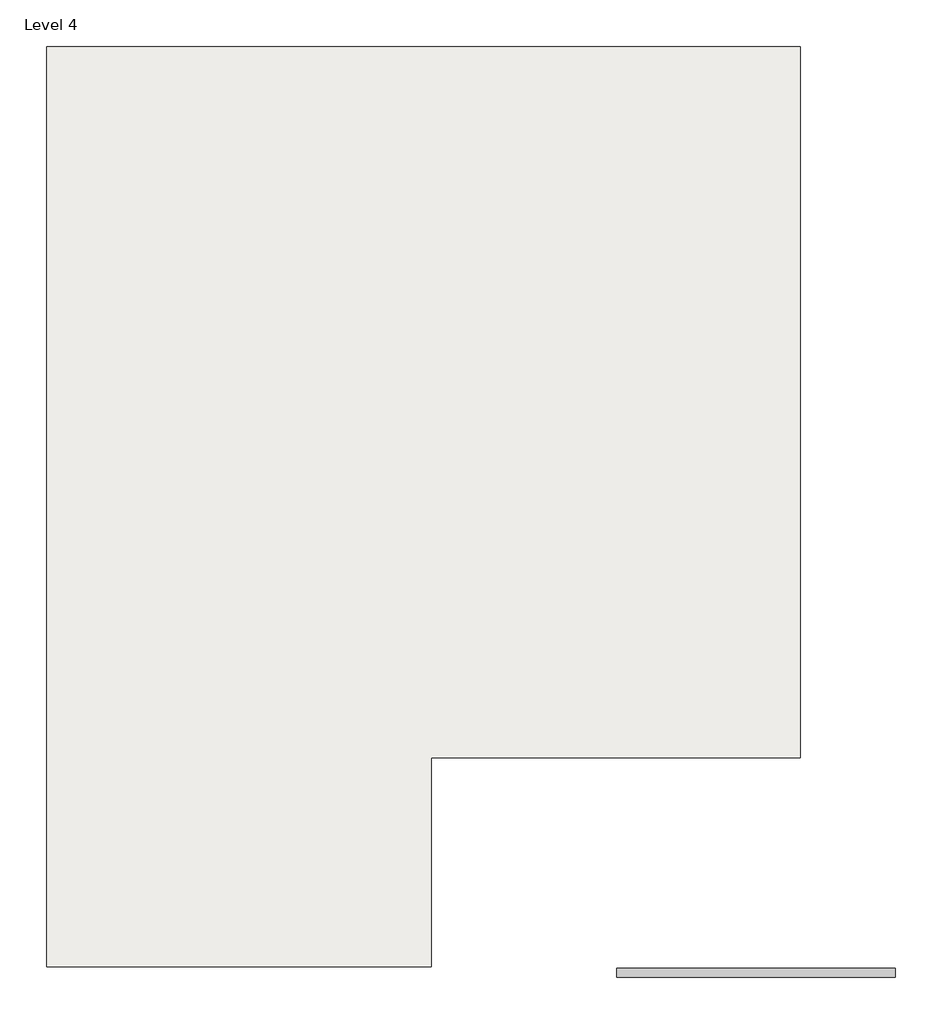
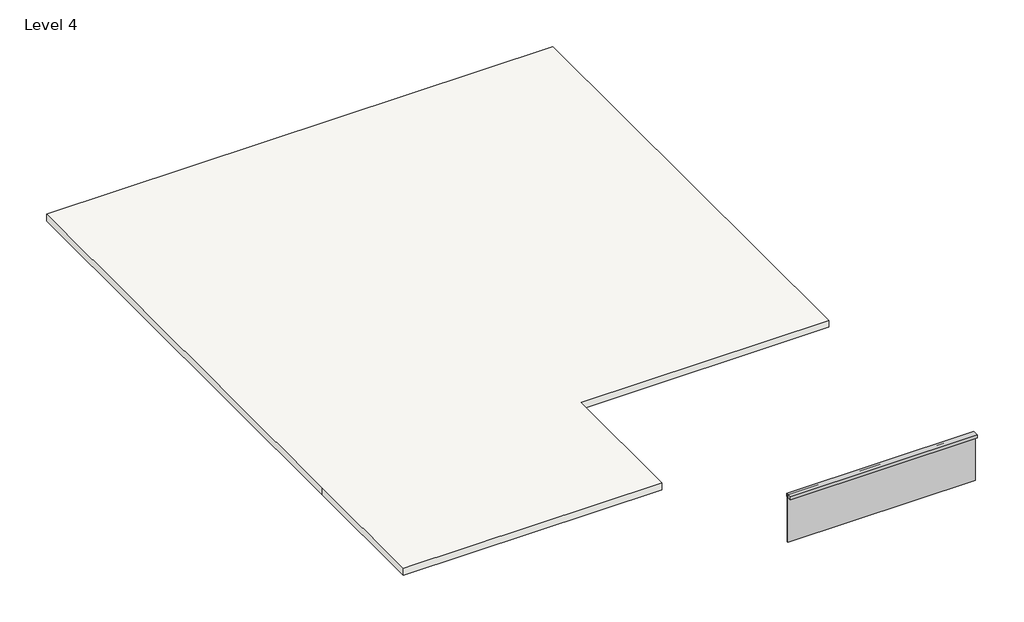
# One storey: 1 member, 1 plate, 1 slab.
"""IFC4 building model written with IfcOpenShell, lengths in millimetres."""

from ifc_helpers import new_model, si_unit, frame, origin, place, context, project, spatial, polyline, outline, extrude, transform, mapped, element, save
from components import member_63be31b3, system_panel_glazed_b77e27d4

model = new_model("IFC4")

# Units and contexts
model_context = context("Model", 3, world=origin())
ifc_project = project(units=[si_unit("LENGTHUNIT", "METRE", prefix="MILLI")], contexts=[model_context])

# Site, building, storey
site = spatial("IfcSite", under=ifc_project)
building = spatial("IfcBuilding", under=site)
storey = spatial("IfcBuildingStorey", under=building, Name="Level 4", Elevation=6858.0)

# Member
placement = place(None, origin())
member_shape = member_63be31b3(model_context)
element("IfcMember", 1, ObjectType="Rectangular Mullion : 2.5\" x 5\" rectangular", at=placement, inside=storey, context=model_context, shape_type="MappedRepresentation", body=[
    mapped(member_shape, transform((2125.7584691, 111.0658856, 5873.8580614), x_axis=(0.0, 0.0, 1.0), y_axis=(0.0, -1.0, 0.0), z_axis=(1.0, 0.0, 0.0))),
])

# Plate
system_panel_glazed_shape = system_panel_glazed_b77e27d4(model_context)
element("IfcPlate", 2, ObjectType="System Panel : Glazed", at=placement, inside=storey, context=model_context, shape_type="MappedRepresentation", body=[
    mapped(system_panel_glazed_shape, transform((169.9584691, 111.0658856, 4819.65), x_axis=(1.0, 0.0, 0.0), y_axis=(0.0, 1.0, 0.0), z_axis=(0.0, 0.0, 1.0))),
])

# Slab
element("IfcSlab", 3, ObjectType="6\"", at=placement, inside=storey, context=model_context, shape_type="SweptSolid", body=[
    extrude(outline(polyline([(793.8459691, 13111.1033856), (793.8459691, 3128.9033856), (-4387.7540309, 3128.9033856), (-4387.7540309, 195.2033856), (-9785.2540309, 195.2033856), (-9785.2540309, 3128.9033856), (-9785.2540309, 13111.1033856), (793.8459691, 13111.1033856)])), frame((0.0, 0.0, 6858.0), z_axis=(0.0, 0.0, 1.0), x_axis=(1.0, 0.0, 0.0)), (0.0, 0.0, 1.0), 152.4),
])

save(model, "model.ifc")

# Revit data of these elements
# Type "Rectangular Mullion : 2.5\" x 5\" rectangular"
#   built-in parameter 1007304 = 0.416667 (stored number, unit not read)
#   built-in parameter 1007301 = 0.104167 (stored number, unit not read)
#   built-in parameter 1007300 = 0.104167 (stored number, unit not read)
# Type "System Panel : Glazed"
#   Construction Type Id = "GSP4R"
#   Analytic Construction = "1/8 in Pilkington single glazing"
#   Visual Light Transmittance = 0.9
#   Solar Heat Gain Coefficient = 0.86
#   Heat Transfer Coefficient (U) = 1.18115 BTU/(h·ft²·°F)
#   Define Thermal Properties by = 1
# Type "6\""
#   Assembly Code = "B1010"
#   Function = 0
#   Layers, outside or top first: 0' - 6" "Gypsum Wall Board" (function 1)
# Element 1 (IfcMember, "Rectangular Mullion : 2.5\" x 5\" rectangular")
#   Phase Created = New Construction
# Element 2 (IfcPlate, "System Panel : Glazed")
#   Phase Created = New Construction
#   Materials on its faces: "Glass"
# Element 3 (IfcSlab, "6\"")
#   Height Offset From Level = 0' - 6"
#   Phase Created = New Construction
#   Materials on its faces: "Gypsum Wall Board"
# Materials
#   "Gypsum Wall Board": class "Generic", colour RGB 127 127 127, transparency 0, Description = "Gypsum Wall Board", Cost = 0
#   "Glass": class "Glass", colour RGB 0 128 192, transparency 0.75, Description = "Soda Lime Glass", Cost = 0
